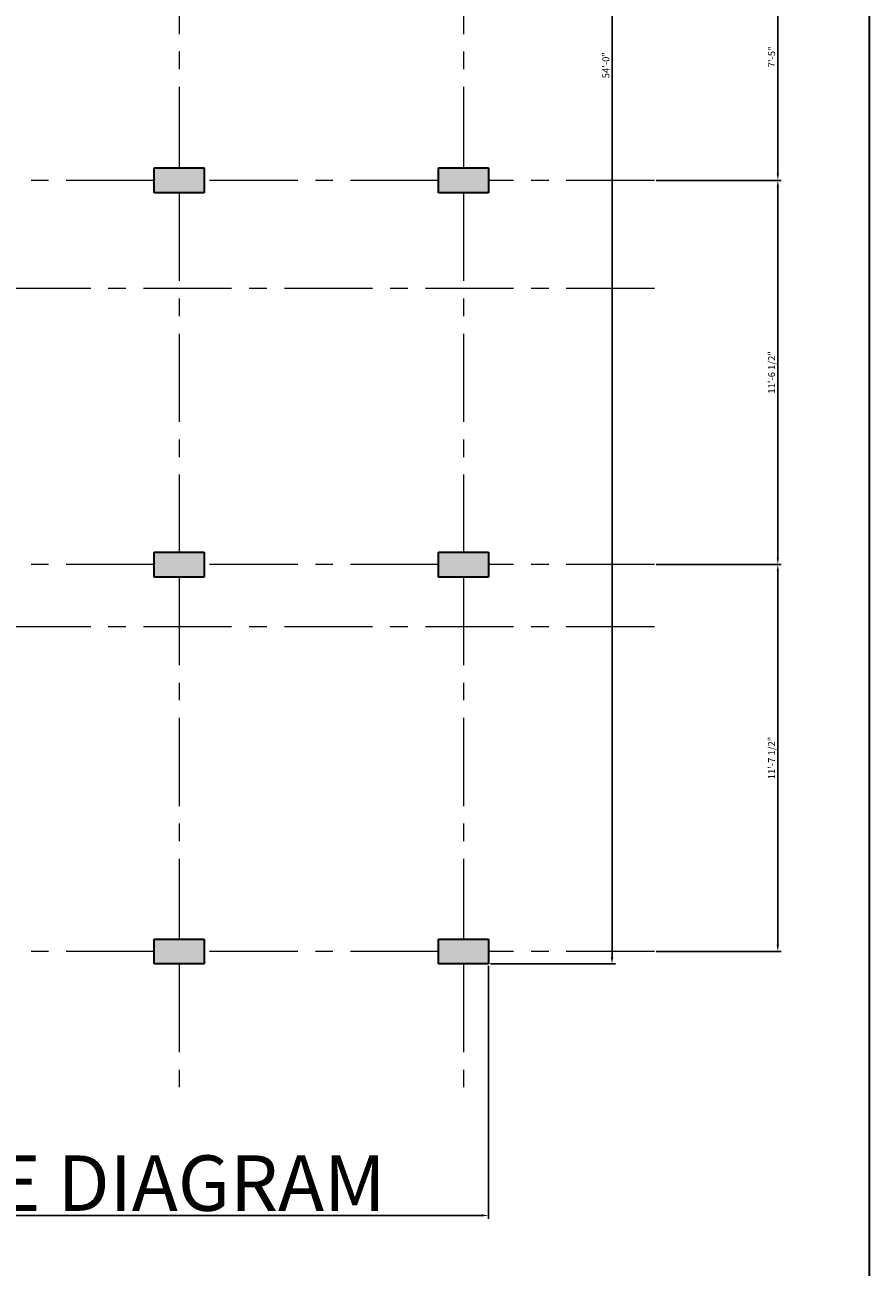
# Model space of a CAD drawing. Units: inches. Extents: x 2391 to 16591, y 7259 to 10239.
# Tile 23 of 27: x 3850 to 4154, y 9245 to 9693. Entities that reach past the tile are written whole.
import ezdxf

# ---------------------------------------------------------------- set-up
doc = ezdxf.new("R2010")
doc.units = ezdxf.units.IN
doc.linetypes.add('CENTER', pattern=[50.8, 31.75, -6.35, 6.35, -6.35])
for name, color, linetype, lineweight in [('A-ANNO-DIMS', 4, 'Continuous', 18), ('A-ANNO-TITL', 3, 'Continuous', 30), ('A-ANNO-TTLB', 7, 'Continuous', 35), ('A-COLS', 3, 'Continuous', 35), ('A-COLS-PATT', 3, 'Continuous', 13), ('A-GRID', 1, 'CENTER', 13)]:
    doc.layers.add(name, color=color, linetype=linetype, lineweight=lineweight)
doc.styles.get("Standard").update_dxf_attribs({"font": 'arial.ttf'})
doc.dimstyles.new('ISO-25', dxfattribs={"dimtxt": 2.5, "dimasz": 2.5, "dimexe": 1.25, "dimexo": 0.625, "dimtad": 1, "dimdec": 0, "dimlunit": 3, "dimtxsty": 'Standard', "dimcen": 2.5, "dimadec": 0, "dimazin": 0, "dimtfac": 1, "dimtdec": 0, "dimtmove": 0, "dimatfit": 3, "dimfxl": 1, "dimarcsym": 0})

# ---------------------------------------------------------------- blocks, each defined once
blk = doc.blocks.new('*D102')
at = {"layer": 'A-ANNO-DIMS', "color": 0, "lineweight": -2, "transparency": 16777216}
for p, q in [((3656.26, 9353.63), (3656.26, 9262.37)), ((4017.01, 9353.63), (4017.01, 9262.37)), ((3658.76, 9263.62), (4014.51, 9263.62))]:
    blk.add_line(p, q, dxfattribs=at)
at = {"layer": 'A-ANNO-DIMS', "color": 0, "transparency": 16777216}
for points in [[(3658.76, 9264.03), (3658.76, 9263.2), (3656.26, 9263.62)], [(4014.51, 9264.03), (4014.51, 9263.2), (4017.01, 9263.62)]]:
    blk.add_solid(points, dxfattribs=at)
at = {"layer": 'Defpoints', "color": 0, "transparency": 16777216}
for p in [(3656.26, 9354.26), (4017.01, 9354.26), (4017.01, 9263.62)]:
    blk.add_point(p, dxfattribs=at)
at = {"layer": 'A-ANNO-DIMS', "color": 0, "transparency": 16777216, "insert": (3836.64, 9265.52), "char_height": 2.5, "attachment_point": 5}
blk.add_mtext('30\'-1"', dxfattribs=at)
blk = doc.blocks.new('*D103')
at = {"layer": 'A-ANNO-DIMS', "color": 0, "lineweight": -2, "transparency": 16777216}
for p, q in [((4017.64, 10002.26), (4062.76, 10002.26)), ((4061.51, 9999.76), (4061.51, 9356.76)), ((4017.64, 9354.26), (4062.76, 9354.26))]:
    blk.add_line(p, q, dxfattribs=at)
at = {"layer": 'A-ANNO-DIMS', "color": 0, "transparency": 16777216}
for points in [[(4061.1, 9999.76), (4061.93, 9999.76), (4061.51, 10002.26)], [(4061.1, 9356.76), (4061.93, 9356.76), (4061.51, 9354.26)]]:
    blk.add_solid(points, dxfattribs=at)
at = {"layer": 'Defpoints', "color": 0, "transparency": 16777216}
for p in [(4017.01, 10002.26), (4017.01, 9354.26), (4061.51, 9354.26)]:
    blk.add_point(p, dxfattribs=at)
at = {"layer": 'A-ANNO-DIMS', "color": 0, "transparency": 16777216, "insert": (4059.61, 9678.26), "char_height": 2.5, "attachment_point": 5, "rotation": 90}
blk.add_mtext('54\'-0"', dxfattribs=at)
blk = doc.blocks.new('*D112')
at = {"layer": 'A-ANNO-DIMS', "color": 0, "lineweight": -2, "transparency": 16777216}
for p, q in [((4077.4, 9498.26), (4122.52, 9498.26)), ((4121.27, 9361.26), (4121.27, 9495.76)), ((4077.4, 9358.76), (4122.52, 9358.76))]:
    blk.add_line(p, q, dxfattribs=at)
at = {"layer": 'A-ANNO-DIMS', "color": 0, "transparency": 16777216}
for points in [[(4120.86, 9495.76), (4121.69, 9495.76), (4121.27, 9498.26)], [(4120.86, 9361.26), (4121.69, 9361.26), (4121.27, 9358.76)]]:
    blk.add_solid(points, dxfattribs=at)
at = {"layer": 'Defpoints', "color": 0, "transparency": 16777216}
for p in [(4076.77, 9498.26), (4121.27, 9498.26), (4076.77, 9358.76)]:
    blk.add_point(p, dxfattribs=at)
at = {"layer": 'A-ANNO-DIMS', "color": 0, "transparency": 16777216, "insert": (4119.36, 9428.51), "char_height": 2.5, "attachment_point": 5, "rotation": 90}
blk.add_mtext('11\'-7 1/2"', dxfattribs=at)
blk = doc.blocks.new('*D113')
at = {"layer": 'A-ANNO-DIMS', "color": 0, "lineweight": -2, "transparency": 16777216}
for p, q in [((4077.4, 9636.76), (4122.52, 9636.76)), ((4121.27, 9500.76), (4121.27, 9634.26)), ((4077.4, 9498.26), (4122.52, 9498.26))]:
    blk.add_line(p, q, dxfattribs=at)
at = {"layer": 'A-ANNO-DIMS', "color": 0, "transparency": 16777216}
for points in [[(4120.86, 9634.26), (4121.69, 9634.26), (4121.27, 9636.76)], [(4120.86, 9500.76), (4121.69, 9500.76), (4121.27, 9498.26)]]:
    blk.add_solid(points, dxfattribs=at)
at = {"layer": 'Defpoints', "color": 0, "transparency": 16777216}
for p in [(4076.77, 9636.76), (4121.27, 9636.76), (4076.77, 9498.26)]:
    blk.add_point(p, dxfattribs=at)
at = {"layer": 'A-ANNO-DIMS', "color": 0, "transparency": 16777216, "insert": (4119.36, 9567.51), "char_height": 2.5, "attachment_point": 5, "rotation": 90}
blk.add_mtext('11\'-6 1/2"', dxfattribs=at)
blk = doc.blocks.new('*D114')
at = {"layer": 'A-ANNO-DIMS', "color": 0, "lineweight": -2, "transparency": 16777216}
for p, q in [((4077.4, 9725.76), (4122.52, 9725.76)), ((4121.27, 9639.26), (4121.27, 9723.26)), ((4077.4, 9636.76), (4122.52, 9636.76))]:
    blk.add_line(p, q, dxfattribs=at)
at = {"layer": 'A-ANNO-DIMS', "color": 0, "transparency": 16777216}
for points in [[(4120.86, 9723.26), (4121.69, 9723.26), (4121.27, 9725.76)], [(4120.86, 9639.26), (4121.69, 9639.26), (4121.27, 9636.76)]]:
    blk.add_solid(points, dxfattribs=at)
at = {"layer": 'Defpoints', "color": 0, "transparency": 16777216}
for p in [(4076.77, 9725.76), (4121.27, 9725.76), (4076.77, 9636.76)]:
    blk.add_point(p, dxfattribs=at)
at = {"layer": 'A-ANNO-DIMS', "color": 0, "transparency": 16777216, "insert": (4119.38, 9681.26), "char_height": 2.5, "attachment_point": 5, "rotation": 90}
blk.add_mtext('7\'-5"', dxfattribs=at)

msp = doc.modelspace()

# ---------------------------------------------------------------- hatches: boundary and pattern name
at = {"layer": 'A-COLS-PATT'}
h = msp.add_hatch(color=256, dxfattribs=at)
h.dxf.hatch_style = 1
h.paths.add_polyline_path([(3674.26, 9993.26), (3674.26, 10002.26), (3656.26, 10002.26), (3656.26, 9993.26)])
h.paths.add_polyline_path([(3777.51, 10002.26), (3777.51, 9993.26), (3795.51, 9993.26), (3795.51, 10002.26)])
h.paths.add_polyline_path([(3896.51, 10002.26), (3896.51, 9993.26), (3914.51, 9993.26), (3914.51, 10002.26)])
h.paths.add_polyline_path([(3999.01, 10002.26), (3999.01, 9993.26), (4017.01, 9993.26), (4017.01, 10002.26)])
h.paths.add_polyline_path([(4017.01, 9860.76), (4017.01, 9869.76), (3999.01, 9869.76), (3999.01, 9860.76)])
h.paths.add_polyline_path([(3914.51, 9860.76), (3914.51, 9869.76), (3896.51, 9869.76), (3896.51, 9860.76)])
h.paths.add_polyline_path([(3777.51, 9885.26), (3777.51, 9876.26), (3795.51, 9876.26), (3795.51, 9885.26)])
h.paths.add_polyline_path([(3674.26, 9876.26), (3674.26, 9885.26), (3656.26, 9885.26), (3656.26, 9876.26)])
h.paths.add_polyline_path([(3656.26, 9766.26), (3656.26, 9757.26), (3674.26, 9757.26), (3674.26, 9766.26)])
h.paths.add_polyline_path([(3786.51, 9759.76), (3795.51, 9759.76), (3795.51, 9777.76), (3786.51, 9777.76)])
h.paths.add_polyline_path([(3914.51, 9721.26), (3914.51, 9730.26), (3896.51, 9730.26), (3896.51, 9721.26)])
h.paths.add_polyline_path([(3999.01, 9730.26), (3999.01, 9721.26), (4017.01, 9721.26), (4017.01, 9730.26)])
h.paths.add_polyline_path([(4017.01, 9632.26), (4017.01, 9641.26), (3999.01, 9641.26), (3999.01, 9632.26)])
h.paths.add_polyline_path([(3914.51, 9632.26), (3914.51, 9641.26), (3896.51, 9641.26), (3896.51, 9632.26)])
h.paths.add_polyline_path([(3795.51, 9632.26), (3786.51, 9632.26), (3786.51, 9614.26), (3795.51, 9614.26)])
h.paths.add_polyline_path([(3656.26, 9602.26), (3656.26, 9593.26), (3674.26, 9593.26), (3674.26, 9602.26)])
h.paths.add_polyline_path([(3674.26, 9471.26), (3674.26, 9480.26), (3656.26, 9480.26), (3656.26, 9471.26)])
h.paths.add_polyline_path([(3795.51, 9489.26), (3786.51, 9489.26), (3786.51, 9471.26), (3795.51, 9471.26)])
h.paths.add_polyline_path([(3896.51, 9502.76), (3896.51, 9493.76), (3914.51, 9493.76), (3914.51, 9502.76)])
h.paths.add_polyline_path([(3999.01, 9502.76), (3999.01, 9493.76), (4017.01, 9493.76), (4017.01, 9502.76)])
h.paths.add_polyline_path([(4017.01, 9354.26), (4017.01, 9363.26), (3999.01, 9363.26), (3999.01, 9354.26)])
h.paths.add_polyline_path([(3914.51, 9354.26), (3914.51, 9363.26), (3896.51, 9363.26), (3896.51, 9354.26)])
h.paths.add_polyline_path([(3795.51, 9354.26), (3795.51, 9363.26), (3777.51, 9363.26), (3777.51, 9354.26)])
h.paths.add_polyline_path([(3674.26, 9354.26), (3674.26, 9363.26), (3656.26, 9363.26), (3656.26, 9354.26)])

# ---------------------------------------------------------------- linework, layer by layer
at = {"layer": 'A-ANNO-TTLB'}
msp.add_lwpolyline([(2391.28, 10239.38), (4154.2, 10239.38), (4154.2, 7258.54), (2391.28, 7258.54)], close=True, dxfattribs=at)
at = {"layer": 'A-COLS'}
for p, q in [((3896.51, 9641.26), (3914.51, 9641.26)), ((3896.51, 9632.26), (3896.51, 9641.26)), ((3914.51, 9641.26), (3914.51, 9632.26)), ((3999.01, 9641.26), (4017.01, 9641.26)), ((3999.01, 9632.26), (3999.01, 9641.26)), ((4017.01, 9641.26), (4017.01, 9632.26)), ((3914.51, 9632.26), (3896.51, 9632.26)), ((4017.01, 9632.26), (3999.01, 9632.26)), ((3896.51, 9502.76), (3914.51, 9502.76)), ((3896.51, 9493.76), (3896.51, 9502.76)), ((3914.51, 9502.76), (3914.51, 9493.76)), ((3999.01, 9502.76), (4017.01, 9502.76)), ((3999.01, 9493.76), (3999.01, 9502.76)), ((4017.01, 9502.76), (4017.01, 9493.76)), ((3914.51, 9493.76), (3896.51, 9493.76)), ((4017.01, 9493.76), (3999.01, 9493.76)), ((3896.51, 9363.26), (3914.51, 9363.26)), ((3896.51, 9354.26), (3896.51, 9363.26)), ((3914.51, 9363.26), (3914.51, 9354.26)), ((3999.01, 9363.26), (4017.01, 9363.26)), ((3999.01, 9354.26), (3999.01, 9363.26)), ((4017.01, 9363.26), (4017.01, 9354.26)), ((3914.51, 9354.26), (3896.51, 9354.26)), ((4017.01, 9354.26), (3999.01, 9354.26))]:
    msp.add_line(p, q, dxfattribs=at)
at = {"layer": 'A-GRID'}
for p, q in [((3905.51, 9721.26), (3905.51, 9641.26)), ((4008.01, 9721.26), (4008.01, 9641.26)), ((3896.51, 9636.76), (3602.07, 9636.76)), ((3999.01, 9636.76), (3914.51, 9636.76)), ((4076.77, 9636.76), (4017.01, 9636.76)), ((3905.51, 9632.26), (3905.51, 9502.76)), ((4008.01, 9632.26), (4008.01, 9502.76)), ((4076.77, 9597.76), (3674.26, 9597.76)), ((4017.01, 9496.26), (4017.01, 9500.26)), ((3896.51, 9498.26), (3602.07, 9498.26)), ((3999.01, 9498.26), (3914.51, 9498.26)), ((4076.77, 9498.26), (4017.01, 9498.26)), ((3905.51, 9493.76), (3905.51, 9363.26)), ((4008.01, 9493.76), (4008.01, 9363.26)), ((4076.77, 9475.76), (3795.51, 9475.76)), ((3896.51, 9358.76), (3795.51, 9358.76)), ((3999.01, 9358.76), (3914.51, 9358.76)), ((4076.77, 9358.76), (4017.01, 9358.76)), ((3905.51, 9354.26), (3905.51, 9308.12)), ((4008.01, 9354.26), (4008.01, 9308.12))]:
    msp.add_line(p, q, dxfattribs=at)

# ---------------------------------------------------------------- texts
at = {"layer": 'A-ANNO-TITL', "insert": (3687.85, 9285.26), "char_height": 20, "attachment_point": 1}
msp.add_mtext_dynamic_manual_height_columns('CENTRE LINE DIAGRAM', width=529.6372, gutter_width=12.5, heights=[0], dxfattribs=at)

# ---------------------------------------------------------------- dimensions: what is measured, and where the dimension line sits
at = {"layer": 'A-ANNO-DIMS'}
for base, p1, p2, angle, picture, middle in [((4061.51, 9354.26), (4017.01, 10002.26), (4017.01, 9354.26), 270, '*D103', (4059.61, 9678.26)), ((4121.27, 9725.76), (4076.77, 9636.76), (4076.77, 9725.76), 90, '*D114', (4119.38, 9681.26)), ((4121.27, 9636.76), (4076.77, 9498.26), (4076.77, 9636.76), 90, '*D113', (4119.36, 9567.51)), ((4121.27, 9498.26), (4076.77, 9358.76), (4076.77, 9498.26), 90, '*D112', (4119.36, 9428.51))]:
    dim = msp.add_linear_dim(base=base, p1=p1, p2=p2, angle=angle, dimstyle='ISO-25', override={"dimdec": 1, "dimlfac": 1, "dimrnd": 0, "dimzin": 1, "dimdsep": 46, "dimlunit": 4, "dimfrac": 2}, dxfattribs=at)
    dim.commit()
    dim.dimension.update_dxf_attribs({"geometry": picture, "text_midpoint": middle})
dim = msp.add_linear_dim(base=(4017.01174, 9263.615693), p1=(3656.26174, 9354.257617), p2=(4017.01174, 9354.257617), dimstyle='ISO-25', override={"dimdec": 1, "dimlfac": 1, "dimrnd": 0, "dimzin": 1, "dimdsep": 46, "dimlunit": 4, "dimfrac": 2}, dxfattribs=at)
dim.commit()
dim.dimension.update_dxf_attribs({"geometry": '*D102', "text_midpoint": (3836.63674, 9265.51797813)})

doc.saveas('drawing.dxf')
